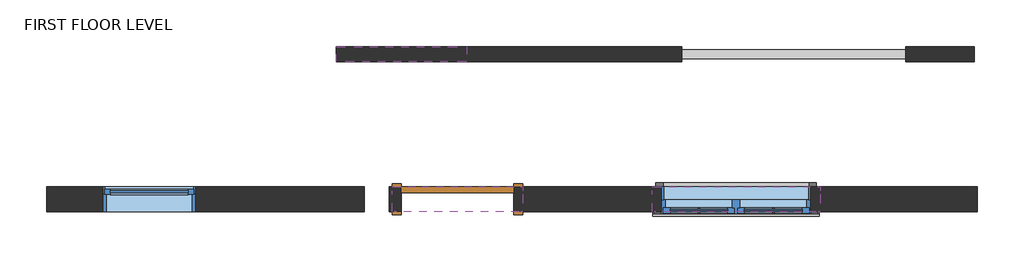
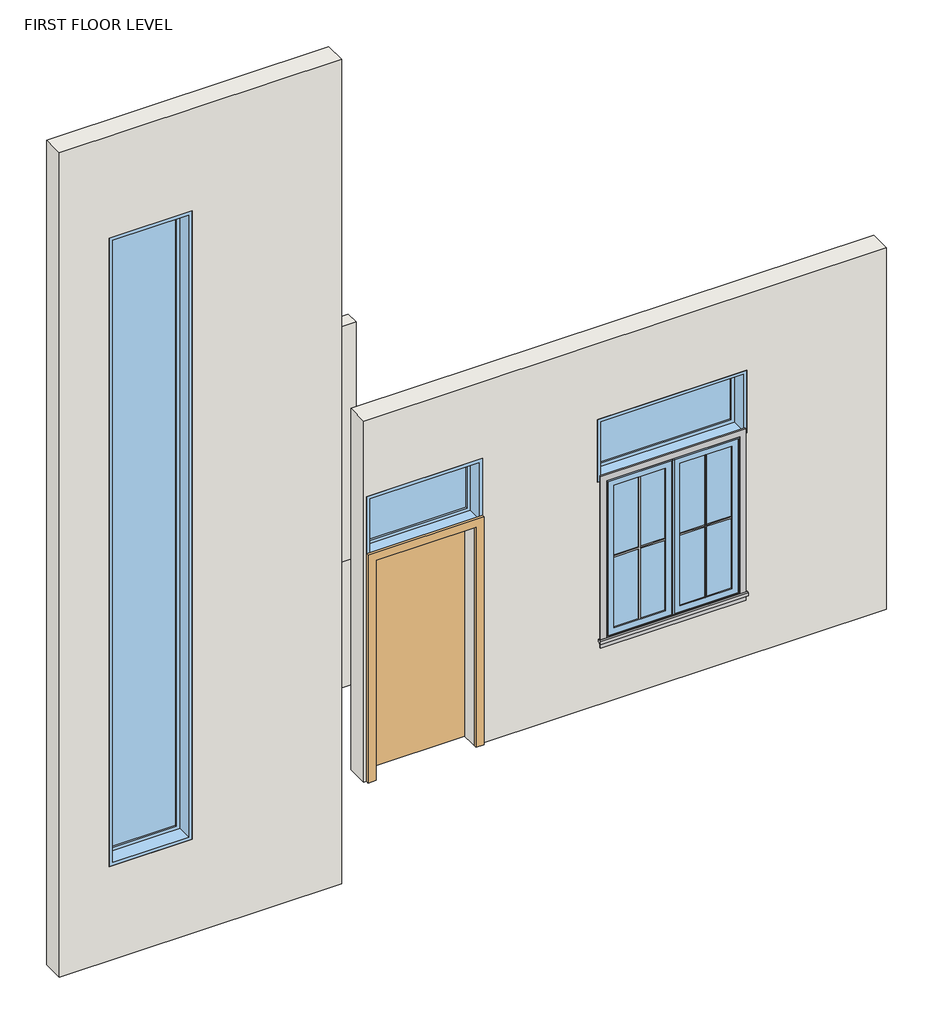
# One storey, incomplete: 4 proxies, 4 walls, 4 windows, 1 door, 1 railing.
"""IFC4 building model written with IfcOpenShell, lengths in millimetres."""

from ifc_helpers import new_model, si_unit, point, frame, origin, place, context, project, spatial, polyline, ellipse_curve, trimmed, outline, extrude, faceted_brep, transform, mapped, element, save
from ifc_brep_helpers import plane_surface, extruded_surface, advanced_brep
from components import muntin_pattern_2x2_muntin_pattern_2x2_6dad3731, muntin_pattern_2x2_muntin_pattern_2x2_a30a3345, trim_window_exterior_flat_with_sill_e3be2e48, trim_window_interior_flat_picture_frame_1906adc9, door_54dd4da4, window_1e0399d0, window_e8893895, window_5b0cf282, window_f2c349b1

model = new_model("IFC4")

# Units and contexts
model_context = context("Model", 3, world=origin())
ifc_project = project(units=[si_unit("LENGTHUNIT", "METRE", prefix="MILLI")], contexts=[model_context])

# Site, building, storey
site = spatial("IfcSite", under=ifc_project)
building = spatial("IfcBuilding", under=site)
storey = spatial("IfcBuildingStorey", under=building, Name="FIRST FLOOR LEVEL", Elevation=4419.6)

# Proxies
placement = place(None, origin())
muntin_pattern_2x2_muntin_pattern_2x2_shape = muntin_pattern_2x2_muntin_pattern_2x2_6dad3731(model_context)
element("IfcBuildingElementProxy", 1, Name="Muntin Pattern_2x2 : Muntin Pattern_2x2", ObjectType="Muntin Pattern_2x2 : Muntin Pattern_2x2", at=placement, inside=storey, context=model_context, shape_type="MappedRepresentation", body=[
    mapped(muntin_pattern_2x2_muntin_pattern_2x2_shape, transform((-13781.656205, -12333.7777976, 5124.45), x_axis=(-1.0, 0.0, 0.0), y_axis=(0.0, -1.0, 0.0), z_axis=(0.0, 0.0, 1.0))),
])
muntin_pattern_2x2_muntin_pattern_2x2_2_shape = muntin_pattern_2x2_muntin_pattern_2x2_a30a3345(model_context)
element("IfcBuildingElementProxy", 2, Name="Muntin Pattern_2x2 : Muntin Pattern_2x2", ObjectType="Muntin Pattern_2x2 : Muntin Pattern_2x2", at=placement, inside=storey, context=model_context, shape_type="MappedRepresentation", body=[
    mapped(muntin_pattern_2x2_muntin_pattern_2x2_2_shape, transform((-14388.081205, -12333.7777976, 5124.45), x_axis=(1.0, 0.0, 0.0), y_axis=(0.0, 1.0, 0.0), z_axis=(0.0, 0.0, 1.0))),
])
trim_window_exterior_flat_with_sill_shape = trim_window_exterior_flat_with_sill_e3be2e48(model_context)
element("IfcBuildingElementProxy", 3, Name="Trim-Window-Exterior-Flat : with Sill", ObjectType="Trim-Window-Exterior-Flat : with Sill", at=placement, inside=storey, context=model_context, shape_type="MappedRepresentation", body=[
    mapped(trim_window_exterior_flat_with_sill_shape, transform((-14084.868705, -12343.3027976, 6578.6), x_axis=(-1.0, 0.0, 0.0), y_axis=(0.0, 0.0, -1.0), z_axis=(0.0, -1.0, 0.0))),
])
trim_window_interior_flat_picture_frame_shape = trim_window_interior_flat_picture_frame_1906adc9(model_context)
element("IfcBuildingElementProxy", 4, Name="Trim-Window-Interior-Flat : Picture Frame", ObjectType="Trim-Window-Interior-Flat : Picture Frame", at=placement, inside=storey, context=model_context, shape_type="MappedRepresentation", body=[
    mapped(trim_window_interior_flat_picture_frame_shape, transform((-14084.868705, -12140.1027976, 6578.6), x_axis=(1.0, 0.0, 0.0), y_axis=(0.0, 0.0, -1.0), z_axis=(0.0, 1.0, 0.0))),
])

# Door
door_shape = door_54dd4da4(model_context)
element("IfcDoor", 5, ObjectType="Single-Flush : 36\" x 84\"", at=placement, inside=storey, context=model_context, shape_type="MappedRepresentation", body=[
    mapped(door_shape, transform((-16358.168705, -12241.7027976, 4419.6), x_axis=(1.0, 0.0, 0.0), y_axis=(0.0, 1.0, 0.0), z_axis=(0.0, 0.0, 1.0))),
])

# Railing
element("IfcRailing", 6, ObjectType="Glass Panel - Bottom Fill", at=placement, inside=storey, context=model_context, shape_type="SolidModel", body=[
    advanced_brep(
    [(-12700.568705, -11097.1152976, 5486.4), (-12700.568705, -11020.9152976, 5486.4), (-14529.368705, -11097.1152976, 5486.4), (-14529.368705, -11020.9152976, 5486.4)],
    [
        (0, 1, ellipse_curve(frame((-12700.568705, -11059.0152976, 5486.4), z_axis=(1.0, 0.0, 0.0), x_axis=(0.0, 1.0, 0.0)), 38.1, 28.575)),
        (1, 0, ellipse_curve(frame((-12700.568705, -11059.0152976, 5486.4), z_axis=(1.0, 0.0, 0.0), x_axis=(0.0, 1.0, 0.0)), 38.1, 28.575)),
        (2, 3, ellipse_curve(frame((-14529.368705, -11059.0152976, 5486.4), z_axis=(-1.0, 0.0, 0.0), x_axis=(0.0, 1.0, 0.0)), 38.1, 28.575)),
        (3, 2, ellipse_curve(frame((-14529.368705, -11059.0152976, 5486.4), z_axis=(-1.0, 0.0, 0.0), x_axis=(0.0, 1.0, 0.0)), 38.1, 28.575)),
        (0, 2),
        (3, 1),
    ],
    [
        plane_surface(frame((-12700.568705, -11059.0152976, 5486.4), z_axis=(1.0, 0.0, 0.0), x_axis=(0.0, -1.0, 0.0))),
        plane_surface(frame((-14529.368705, -11059.0152976, 5486.4), z_axis=(-1.0, 0.0, 0.0), x_axis=(0.0, -1.0, 0.0))),
        extruded_surface(trimmed(ellipse_curve(frame((-14529.368705, -11059.0152976, 5486.4), z_axis=(1.0, 0.0, 0.0), x_axis=(0.0, 1.0, 0.0)), 38.1, 28.575), [point((-14529.368705, -11097.1152976, 5486.4))], [point((-14529.368705, -11020.9152976, 5486.4))], True, "CARTESIAN"), (1828.800000000001, 0.0, 0.0), 1828.800000000001),
        extruded_surface(trimmed(ellipse_curve(frame((-14529.368705, -11059.0152976, 5486.4), z_axis=(1.0, 0.0, 0.0), x_axis=(0.0, 1.0, 0.0)), 38.1, 28.575), [point((-14529.368705, -11020.9152976, 5486.4))], [point((-14529.368705, -11097.1152976, 5486.4))], True, "CARTESIAN"), (1828.800000000001, 0.0, 0.0), 1828.800000000001),
    ],
    [
        (0, [[1, 2]]),
        (1, [[3, 4]]),
        (2, [[-1, 5, -4, 6]]),
        (3, [[-2, -6, -3, -5]]),
    ],
),
    extrude(outline(polyline([(-12700.568705, -11046.3152976), (-12700.568705, -11071.7152976), (-14529.368705, -11071.7152976), (-14529.368705, -11046.3152976), (-12700.568705, -11046.3152976)])), frame((0.0, 0.0, 5372.1), z_axis=(0.0, 0.0, 1.0), x_axis=(1.0, 0.0, 0.0)), (0.0, 0.0, 1.0), 25.4),
    extrude(outline(polyline([(-12700.568705, -11046.3152976), (-12700.568705, -11071.7152976), (-14529.368705, -11071.7152976), (-14529.368705, -11046.3152976), (-12700.568705, -11046.3152976)])), frame((0.0, 0.0, 5270.5), z_axis=(0.0, 0.0, 1.0), x_axis=(1.0, 0.0, 0.0)), (0.0, 0.0, 1.0), 25.4),
    extrude(outline(polyline([(-14421.418705, -11033.6152976), (-14421.418705, -11084.4152976), (-14434.118705, -11084.4152976), (-14434.118705, -11033.6152976), (-14421.418705, -11033.6152976)])), frame((0.0, 0.0, 4572.0), z_axis=(0.0, 0.0, 1.0), x_axis=(1.0, 0.0, 0.0)), (0.0, 0.0, 1.0), 885.825),
    extrude(outline(polyline([(-13614.968705, -11065.5504546), (-14427.768705, -11065.5504546), (-14427.768705, -11059.2004546), (-13614.968705, -11059.2004546), (-13614.968705, -11065.5504546)])), frame((0.0, 0.0, 4673.6), z_axis=(0.0, 0.0, 1.0), x_axis=(1.0, 0.0, 0.0)), (0.0, 0.0, 1.0), 596.9),
    extrude(outline(polyline([(-13608.618705, -11033.6152976), (-13608.618705, -11084.4152976), (-13621.318705, -11084.4152976), (-13621.318705, -11033.6152976), (-13608.618705, -11033.6152976)])), frame((0.0, 0.0, 4572.0), z_axis=(0.0, 0.0, 1.0), x_axis=(1.0, 0.0, 0.0)), (0.0, 0.0, 1.0), 885.825),
    extrude(outline(polyline([(-12802.168705, -11065.5504546), (-13614.968705, -11065.5504546), (-13614.968705, -11059.2004546), (-12802.168705, -11059.2004546), (-12802.168705, -11065.5504546)])), frame((0.0, 0.0, 4673.6), z_axis=(0.0, 0.0, 1.0), x_axis=(1.0, 0.0, 0.0)), (0.0, 0.0, 1.0), 596.9),
    extrude(outline(polyline([(-12795.818705, -11033.6152976), (-12795.818705, -11084.4152976), (-12808.518705, -11084.4152976), (-12808.518705, -11033.6152976), (-12795.818705, -11033.6152976)])), frame((0.0, 0.0, 4572.0), z_axis=(0.0, 0.0, 1.0), x_axis=(1.0, 0.0, 0.0)), (0.0, 0.0, 1.0), 885.825),
    extrude(outline(polyline([(-14516.668705, -11049.4902976), (-14516.668705, -11068.5402976), (-14535.718705, -11068.5402976), (-14535.718705, -11049.4902976), (-14516.668705, -11049.4902976)])), frame((0.0, 0.0, 4572.0), z_axis=(0.0, 0.0, 1.0), x_axis=(1.0, 0.0, 0.0)), (0.0, 0.0, 1.0), 885.825),
    extrude(outline(polyline([(-12694.218705, -11049.4902976), (-12694.218705, -11068.5402976), (-12713.268705, -11068.5402976), (-12713.268705, -11049.4902976), (-12694.218705, -11049.4902976)])), frame((0.0, 0.0, 4572.0), z_axis=(0.0, 0.0, 1.0), x_axis=(1.0, 0.0, 0.0)), (0.0, 0.0, 1.0), 885.825),
])

# Walls
element("IfcWall", 7, ObjectType="Generic - 8\"", at=placement, inside=storey, context=model_context, shape_type="Brep", body=[
    faceted_brep([(-17120.168705, -12140.1027976, 3505.2), (-19710.968705, -12140.1027976, 3505.2), (-19710.968705, -12140.1027976, 11506.2), (-17120.168705, -12140.1027976, 11506.2), (-17120.168705, -12140.1027976, 7924.8), (-17120.168705, -12140.1027976, 4419.6), (-18491.768705, -12140.1027976, 10515.6), (-19253.768705, -12140.1027976, 10515.6), (-19253.768705, -12140.1027976, 4419.6), (-18491.768705, -12140.1027976, 4419.6), (-17120.168705, -12343.3027976, 3505.2), (-17120.168705, -12343.3027976, 4419.6), (-17120.168705, -12343.3027976, 11506.2), (-19710.968705, -12343.3027976, 11506.2), (-19710.968705, -12343.3027976, 3505.2), (-18491.768705, -12343.3027976, 10515.6), (-18491.768705, -12343.3027976, 4419.6), (-19253.768705, -12343.3027976, 4419.6), (-19253.768705, -12343.3027976, 10515.6)], [[[0, 1, 2, 3, 4, 5], [6, 7, 8, 9]], [[10, 11, 12, 13, 14], [15, 16, 17, 18]], [[1, 0, 10, 14]], [[2, 1, 14, 13]], [[3, 2, 13, 12]], [[16, 15, 6, 9]], [[17, 16, 9, 8]], [[18, 17, 8, 7]], [[15, 18, 7, 6]], [[0, 5, 4, 3, 12, 11, 10]]]),
])
element("IfcWall", 8, ObjectType="Generic - 8\" 2", at=placement, inside=storey, context=model_context, shape_type="SweptSolid", body=[
    extrude(outline(polyline([(7924.8, -12116.368705), (7924.8, -16916.968705), (4419.6, -16916.968705), (4419.6, -16815.368705), (6553.2, -16815.368705), (6553.2, -15900.968705), (4419.6, -15900.968705), (4419.6, -12116.368705), (7924.8, -12116.368705)]), holes=[polyline([(7181.85, -15824.768705), (6572.25, -15824.768705), (6572.25, -16891.568705), (7181.85, -16891.568705), (7181.85, -15824.768705)]), polyline([(7188.2, -13399.068705), (6578.6, -13399.068705), (6578.6, -13475.268705), (5054.6, -13475.268705), (5054.6, -14694.468705), (6578.6, -14694.468705), (6578.6, -14770.668705), (7188.2, -14770.668705), (7188.2, -13399.068705)])]), frame((0.0, -12343.3027976, 0.0), z_axis=(0.0, 1.0, 0.0), x_axis=(0.0, 0.0, 1.0)), (0.0, 0.0, 1.0), 203.2),
])
element("IfcWall", 9, ObjectType="Interior - 4 7/8\" Partition (1-hr) 2", at=placement, inside=storey, context=model_context, shape_type="Brep", body=[
    faceted_brep([(-12141.768705, -11120.9277976, 4419.6), (-12141.768705, -11120.9277976, 5638.8), (-12700.568705, -11120.9277976, 5638.8), (-12700.568705, -11120.9277976, 4419.6), (-12141.768705, -10997.1027976, 5638.8), (-12141.768705, -10997.1027976, 4419.6), (-12700.568705, -10997.1027976, 4419.6), (-12700.568705, -10997.1027976, 5638.8)], [[[0, 1, 2, 3]], [[4, 5, 6, 7]], [[5, 0, 3, 6]], [[1, 0, 5, 4]], [[1, 4, 7, 2]], [[3, 2, 7, 6]]]),
    faceted_brep([(-17348.768705, -11120.9277976, 5638.8), (-17348.768705, -11120.9277976, 4419.6), (-14529.368705, -11120.9277976, 4419.6), (-14529.368705, -11120.9277976, 5638.8), (-16281.968705, -11120.9277976, 5638.8), (-17348.768705, -10997.1027976, 4419.6), (-17348.768705, -10997.1027976, 5638.8), (-16281.968705, -10997.1027976, 5638.8), (-14529.368705, -10997.1027976, 5638.8), (-14529.368705, -10997.1027976, 4419.6)], [[[0, 1, 2, 3, 4]], [[5, 6, 7, 8, 9]], [[1, 5, 9, 2]], [[6, 0, 4, 3, 8, 7]], [[1, 0, 6, 5]], [[3, 2, 9, 8]]]),
])
element("IfcWall", 10, ObjectType="Interior - 4 7/8\" Partition (1-hr) 2", at=placement, inside=storey, context=model_context, shape_type="SweptSolid", body=[
    extrude(outline(polyline([(5638.8, -17348.768705), (5638.8, -16281.968705), (7924.8, -16281.968705), (7924.8, -17348.768705), (5638.8, -17348.768705)]), holes=[polyline([(7737.0096329, -17200.5652179), (7737.0096329, -16436.9016135), (5751.8986733, -16436.9016135), (5751.8986733, -17200.5652179), (7737.0096329, -17200.5652179)])]), frame((0.0, -11120.9277976, 0.0), z_axis=(0.0, 1.0, 0.0), x_axis=(0.0, 0.0, 1.0)), (0.0, 0.0, 1.0), 123.825),
])

# Windows
window_shape = window_1e0399d0(model_context)
element("IfcWindow", 11, ObjectType="Fixed : 30\" x 240\"", at=placement, inside=storey, context=model_context, shape_type="MappedRepresentation", body=[
    mapped(window_shape, transform((-18834.668705, -12241.7027976, 3505.2), x_axis=(1.0, 0.0, 0.0), y_axis=(0.0, 1.0, 0.0), z_axis=(0.0, 0.0, 1.0))),
])
window_2_shape = window_e8893895(model_context)
element("IfcWindow", 12, ObjectType="Fixed : 42\" x 24\"", at=placement, inside=storey, context=model_context, shape_type="MappedRepresentation", body=[
    mapped(window_2_shape, transform((-16320.068705, -12241.7027976, 4438.65), x_axis=(1.0, 0.0, 0.0), y_axis=(0.0, 1.0, 0.0), z_axis=(0.0, 0.0, 1.0))),
])
window_3_shape = window_5b0cf282(model_context)
element("IfcWindow", 13, ObjectType="Fixed : 54\" x 24\"", at=placement, inside=storey, context=model_context, shape_type="MappedRepresentation", body=[
    mapped(window_3_shape, transform((-14046.768705, -12241.7027976, 4445.0), x_axis=(1.0, 0.0, 0.0), y_axis=(0.0, 1.0, 0.0), z_axis=(0.0, 0.0, 1.0))),
])
window_4_shape = window_f2c349b1(model_context)
element("IfcWindow", 14, ObjectType="Window-Casement-Double : 48\" x 60\"", at=placement, inside=storey, context=model_context, shape_type="MappedRepresentation", body=[
    mapped(window_4_shape, transform((-14084.868705, -12241.7027976, 4140.2), x_axis=(1.0, 0.0, 0.0), y_axis=(0.0, 1.0, 0.0), z_axis=(0.0, 0.0, 1.0))),
])

save(model, "model.ifc")

# Revit data of these elements
# Type "Muntin Pattern_2x2 : Muntin Pattern_2x2"
#   Width [instance default] = 4' - 0"
#   Thickness = 0' - 0 1/2"
#   Height [instance default] = 4' - 0"
#   Distance = 0' - 0 3/4"
#   Interior Material [instance default] = none
#   Exterior Material [instance default] = none
#   Default Elevation = 0
# Type "Trim-Window-Exterior-Flat : with Sill"
#   Trim Width = 0' - 2 1/4"
#   Trim Thickness_Picture Frame = 0' - 1 1/4"
#   Trim Thickness_with Sill = 0' - 0 3/4"
#   Sill Thickness = 0' - 1 1/4"
#   Opening Width [instance default] = 2' - 0"
#   Opening Height [instance default] = 3' - 0"
#   Default Elevation = 4' - 0"
#   Sill = yes
#   Picture Frame = no
#   Trim Material [instance default] = none
# Type "Trim-Window-Interior-Flat : Picture Frame"
#   Trim Thickness_Picture Frame = 0' - 1 1/4"
#   Trim Width = 0' - 2 1/4"
#   Trim Thickness_with Sill = 0' - 0 3/4"
#   Sill Thickness = 0' - 1 1/4"
#   Opening Width [instance default] = 2' - 0"
#   Opening Height [instance default] = 3' - 0"
#   Default Elevation = 4' - 0"
#   Sill = no
#   Picture Frame = yes
#   Trim Material [instance default] = none
# Type "Single-Flush : 36\" x 84\""
#   Type Mark = "1"
#   Construction Type Id = "MDOOR"
#   Assembly Code = "C1020"
#   Analytic Construction = "Metal"
#   Thickness = 0' - 2"
#   Heat Transfer Coefficient (U) = 0.651978 BTU/(h·ft²·°F)
#   Height = 7' - 0"
#   Trim Projection Ext = 0' - 1"
#   Trim Projection Int = 0' - 1"
#   Trim Width = 0' - 3"
#   Width = 3' - 0"
#   Define Thermal Properties by = 1
#   Define Thermal Properties by = 1
#   Door Material = Door - Panel
#   Frame Material = Door - Frame
#   Visual Light Transmittance = 0
#   Solar Heat Gain Coefficient = 0
#   Function = (empty or 0)
#   Wall Closure = (empty or 0)
# Type "Glass Panel - Bottom Fill"
#   Assembly Code = "C2010400"
#   built-in parameter 1008612 = 0.0416667 (stored number, unit not read)
#   built-in parameter 1008611 = 0.0416667 (stored number, unit not read)
#   built-in parameter 1008609 = 0.333333 (stored number, unit not read)
#   built-in parameter 1008604 = 0.166667 (stored number, unit not read)
#   built-in parameter 1008603 = 0.166667 (stored number, unit not read)
#   Railing Height = 3' - 0"
#   built-in parameter 1008630 = 2
#   built-in parameter 1008610 = 2
#   built-in parameter 1008618 = Baluster - Square : 3/4"
# Type "Generic - 8\""
#   Assembly Code = "B2010"
#   Layers, outside or top first: 0' - 8" no material (function 1)
# Type "Generic - 8\" 2"
#   Assembly Code = "B2010"
# Type "Interior - 4 7/8\" Partition (1-hr) 2"
#   Assembly Code = "C1010145"
# Type "Fixed : 30\" x 240\""
#   Type Mark = "21"
#   Construction Type Id = "GSP4R"
#   Assembly Code = "B2020100"
#   Analytic Construction = "1/8 in Pilkington single glazing"
#   Visual Light Transmittance = 0.9
#   Solar Heat Gain Coefficient = 0.78
#   Heat Transfer Coefficient (U) = 0.6496 BTU/(h·ft²·°F)
#   Height = 20' - 0"
#   Default Sill Height = 3' - 0"
#   Width = 2' - 6"
#   Window Inset = 0' - 0 3/4"
#   Define Thermal Properties by = 1
#   Glass Pane Material = Glass
#   Sash Material = Damp-proofing
#   Wall Closure = (empty or 0)
# Type "Fixed : 42\" x 24\""
#   Type Mark = "18"
#   Construction Type Id = "GSP4R"
#   Assembly Code = "B2020100"
#   Analytic Construction = "1/8 in Pilkington single glazing"
#   Visual Light Transmittance = 0.9
#   Solar Heat Gain Coefficient = 0.78
#   Heat Transfer Coefficient (U) = 0.6496 BTU/(h·ft²·°F)
#   Height = 2' - 0"
#   Default Sill Height = 7' - 0"
#   Width = 3' - 6"
#   Window Inset = 0' - 0 3/4"
#   Define Thermal Properties by = 1
#   Glass Pane Material = Glass
#   Sash Material = Sash
#   Wall Closure = (empty or 0)
# Type "Fixed : 54\" x 24\""
#   Type Mark = "20"
#   Construction Type Id = "GSP4R"
#   Assembly Code = "B2020100"
#   Analytic Construction = "1/8 in Pilkington single glazing"
#   Visual Light Transmittance = 0.9
#   Solar Heat Gain Coefficient = 0.78
#   Heat Transfer Coefficient (U) = 0.6496 BTU/(h·ft²·°F)
#   Height = 2' - 0"
#   Default Sill Height = 7' - 0"
#   Width = 4' - 6"
#   Window Inset = 0' - 0 3/4"
#   Define Thermal Properties by = 1
#   Glass Pane Material = Glass
#   Sash Material = Sash
#   Wall Closure = (empty or 0)
# Type "Window-Casement-Double : 48\" x 60\""
#   Type Mark = "16"
#   Fire Rating = "0.5h"
#   Assembly Code = "B2020100"
#   Analytic Construction = "Double glazing - domestic"
#   Frame Extension [instance default] = 0' - 0 1/4"
#   Window Inset [instance default] = 0' - 0"
#   Wall Thickness [instance default] = 0' - 6"
#   Interior Wall Closure [instance default] = 0' - 2 1/4"
#   Half Width = 2' - 0"
#   Visual Light Transmittance = 0.81
#   Thermal Resistance (R) = 1.8146 (h·ft²·°F)/BTU
#   Solar Heat Gain Coefficient = 0.76
#   Rough Width = 4' - 0 1/2"
#   Rough Height = 5' - 0 1/2"
#   Height = 5' - 0"
#   Heat Transfer Coefficient (U) = 0.5511 BTU/(h·ft²·°F)
#   Exterior Wall Closure [instance default] = 0' - 1 1/4"
#   Extension Jamb [instance default] = 0' - 2 1/4"
#   Default Sill Height = 3' - 0"
#   Width = 4' - 0"
#   Define Thermal Properties by = 0
#   Muntin Visibility = yes
#   Interior Trim Visibility [instance default] = yes
#   Exterior Trim Visibility [instance default] = yes
#   Extension Jamb Visibility [instance default] = yes
#   Interior Trim Material = Wood - Stained
#   Muntin Pattern = Muntin Pattern_2x2 : Muntin Pattern_2x2
#   Interior Trim = Trim-Window-Interior-Flat : Picture Frame
#   Interior Frame Material = Wood - Stained
#   Glass Panel Material = Glass
#   Exterior Trim Material = Clad - White
#   Exterior Trim = Trim-Window-Exterior-Flat : with Sill
#   Exterior Frame Material = Clad - White
#   Wall Closure = (empty or 0)
# Elements 1, 2 (IfcBuildingElementProxy, "Muntin Pattern_2x2 : Muntin Pattern_2x2")
#   Width = 1' - 6 5/8"
#   Height = 4' - 6 1/2"
#   Interior Material = Wood - Stained
#   Exterior Material = Clad - White
#   Phase Created = New Construction
#   Materials on its faces: "Clad - White", "Wood - Stained"
# Element 3 (IfcBuildingElementProxy, "Trim-Window-Exterior-Flat : with Sill")
#   Opening Width = 4' - 0"
#   Opening Height = 5' - 0"
#   Trim Material = Clad - White
#   Phase Created = New Construction
#   Materials on its faces: "Clad - White"
# Element 4 (IfcBuildingElementProxy, "Trim-Window-Interior-Flat : Picture Frame")
#   Opening Width = 4' - 0"
#   Opening Height = 5' - 0"
#   Trim Material = Wood - Stained
#   Phase Created = New Construction
#   Materials on its faces: "Wood - Stained"
# Element 5 (IfcDoor, "Single-Flush : 36\" x 84\"")
#   Phase Created = New Construction
#   Materials on its faces: "Door - Frame", "Door - Panel"
# Element 6 (IfcRailing, "Glass Panel - Bottom Fill")
#   built-in parameter 1008621 = 0.5 (stored number, unit not read)
#   Phase Created = New Construction
#   Materials on its faces: "Glass"
# Element 7 (IfcWall, "Generic - 8\"")
#   built-in parameter 1001111 = -3' - 0"
#   Top Offset = 0' - 0"
#   Base Offset = -3' - 0"
#   wall height = 26' - 3"
#   Phase Created = New Construction
#   Base Constraint = FIRST FLOOR LEVEL
#   Top Constraint = TOP LEVEL
#   Materials on its faces: "Default Wall"
# Element 8 (IfcWall, "Generic - 8\" 2")
#   Top Offset = 0' - 0"
#   Base Offset = 0' - 0"
#   wall height = 11' - 6"
#   Phase Created = New Construction
#   Base Constraint = FIRST FLOOR LEVEL
#   Top Constraint = ROOF LEVEL
# Element 9 (IfcWall, "Interior - 4 7/8\" Partition (1-hr) 2")
#   Top Offset = 0' - 0"
#   Base Offset = 0' - 0"
#   Unconnected Height = 4' - 0"
#   wall height = 4' - 0"
#   Phase Created = New Construction
#   Base Constraint = FIRST FLOOR LEVEL
#   Materials on its faces: "Default Wall", "Gypsum Wall Board"
# Element 10 (IfcWall, "Interior - 4 7/8\" Partition (1-hr) 2")
#   built-in parameter 1001111 = 4' - 0"
#   Top Offset = 0' - 0"
#   Base Offset = 4' - 0"
#   wall height = 7' - 6"
#   Phase Created = New Construction
#   Base Constraint = FIRST FLOOR LEVEL
#   Top Constraint = ROOF LEVEL
#   Materials on its faces: "Default Wall", "Gypsum Wall Board"
# Element 11 (IfcWindow, "Fixed : 30\" x 240\"")
#   Mark = "6"
#   Phase Created = New Construction
#   Materials on its faces: "Damp-proofing", "Glass"
# Element 12 (IfcWindow, "Fixed : 42\" x 24\"")
#   Mark = "7"
#   Phase Created = New Construction
#   Materials on its faces: "Sash", "Glass"
# Element 13 (IfcWindow, "Fixed : 54\" x 24\"")
#   Mark = "8"
#   Phase Created = New Construction
#   Materials on its faces: "Sash", "Glass"
# Element 14 (IfcWindow, "Window-Casement-Double : 48\" x 60\"")
#   Mark = "9"
#   Window Inset = 0' - 0"
#   Interior Wall Closure = 0' - 2 1/4"
#   Frame Extension = 0' - 0 1/4"
#   Exterior Wall Closure = 0' - 1 1/4"
#   Interior Trim Visibility = yes
#   Exterior Trim Visibility = yes
#   Phase Created = New Construction
#   Materials on its faces: "Wood - Stained", "Glass", "Clad - White"
# Materials
#   "Door - Panel": class "Wood", colour RGB 210 159 95, transparency 0, Cost = 0
#   "Door - Frame": colour RGB 118 70 51, transparency 0, Cost = 0
#   "Glass": class "Glass", colour RGB 0 128 192, transparency 0.75, Description = "Soda Lime Glass", Cost = 0
#   "Damp-proofing": class "Generic", colour RGB 17 17 17, transparency 0, Description = "Damp-proofing", Cost = 0
#   "Sash": class "Wood", colour RGB 224 178 126, transparency 0, Cost = 0
#   "Wood - Stained": class "Wood", colour RGB 224 178 126, transparency 0, Cost = 0
#   "Clad - White": class "Wood", colour RGB 242 242 238, transparency 0, Cost = 0
#   "Default Wall": colour RGB 128 128 128, transparency 0, Cost = 0
#   "Gypsum Wall Board": class "Generic", colour RGB 228 228 228, transparency 0, Description = "Gypsum Wall Board", Cost = 0
